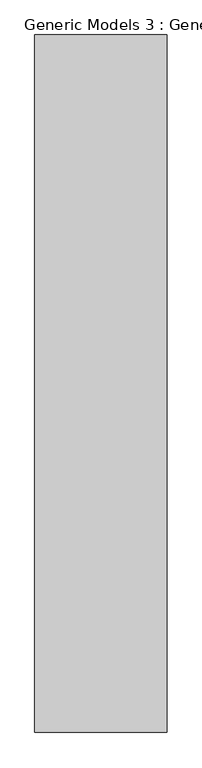
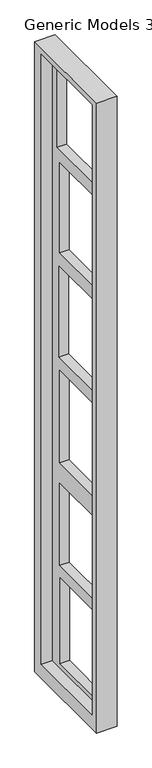
"""IFC4 building model written with IfcOpenShell, lengths in millimetres: proxy geometry, Generic Models 3 : Generic Models 1."""

from ifc_helpers import new_model, si_unit, origin, place, context, project, spatial, faceted_brep, source, transform, mapped, element, save


def generic_models_3_generic_models_1_639dc579(model_context):
    return source(origin(), model_context, "Body", "Brep", [
        faceted_brep([(-6457.5487703, -529.1037749, 18288.0), (-6457.5487703, 2442.6962251, 18288.0), (-7022.5256993, 2442.6962251, 18288.0), (-7022.5256993, -529.1037749, 18288.0), (-6457.5487703, -529.1037749, -158.4213758), (-7022.5256993, -529.1037749, -158.4213758), (-7022.5256993, 2442.6962251, -158.4213758), (-6457.5487703, 2442.6962251, -158.4213758), (-6457.5487703, 80.4962251, 15427.4465317), (-6457.5487703, 80.4962251, 17896.0910797), (-6457.5487703, 1889.1429371, 17896.0910797), (-6457.5487703, 1889.1429371, 15427.4465317), (-6457.5487703, -8.6872134, 12397.0580072), (-6457.5487703, -8.6872134, 15042.3231805), (-6457.5487703, 1781.5076359, 15042.3231805), (-6457.5487703, 1781.5076359, 12397.0580072), (-6457.5487703, -17.3853235, 9328.6434489), (-6457.5487703, -17.3853235, 11990.9234937), (-6457.5487703, 1807.8390259, 11990.9234937), (-6457.5487703, 1807.8390259, 9328.6434489), (-6457.5487703, -30.6801441, 6248.4), (-6457.5487703, -30.6801441, 8955.1024994), (-6457.5487703, 1778.1125113, 8955.1024994), (-6457.5487703, 1778.1125113, 6248.4), (-6457.5487703, -22.1772395, 3249.0844472), (-6457.5487703, -22.1772395, 5661.4894523), (-6457.5487703, 1769.7396662, 5661.4894523), (-6457.5487703, 1769.7396662, 3249.0844472), (-6457.5487703, -35.8456262, 382.1575328), (-6457.5487703, -35.8456262, 2893.6398867), (-6457.5487703, 1759.3912226, 2893.6398867), (-6457.5487703, 1759.3912226, 382.1575328), (-7022.5256993, -312.6392341, 18107.7487565), (-7022.5256993, -312.6392341, 247.1582995), (-7022.5256993, 2127.9635925, 247.1582995), (-7022.5256993, 2127.9635925, 18107.7487565), (-6717.7256993, -312.6392341, 18107.7487565), (-6717.7256993, 2127.9635925, 18107.7487565), (-6717.7256993, 2127.9635925, 247.1582995), (-6717.7256993, -312.6392341, 247.1582995), (-6717.7256993, 80.4962251, 17896.0910797), (-6717.7256993, 80.4962251, 15427.4465317), (-6717.7256993, 1889.1429371, 15427.4465317), (-6717.7256993, 1889.1429371, 17896.0910797), (-6717.7256993, -8.6872134, 15042.3231805), (-6717.7256993, -8.6872134, 12397.0580072), (-6717.7256993, 1781.5076359, 12397.0580072), (-6717.7256993, 1781.5076359, 15042.3231805), (-6717.7256993, -17.3853235, 11990.9234937), (-6717.7256993, -17.3853235, 9328.6434489), (-6717.7256993, 1807.8390259, 9328.6434489), (-6717.7256993, 1807.8390259, 11990.9234937), (-6717.7256993, -30.6801441, 8955.1024994), (-6717.7256993, -30.6801441, 6248.4), (-6717.7256993, 1778.1125113, 6248.4), (-6717.7256993, 1778.1125113, 8955.1024994), (-6717.7256993, -22.1772395, 5661.4894523), (-6717.7256993, -22.1772395, 3249.0844472), (-6717.7256993, 1769.7396662, 3249.0844472), (-6717.7256993, 1769.7396662, 5661.4894523), (-6717.7256993, -35.8456262, 2893.6398867), (-6717.7256993, -35.8456262, 382.1575328), (-6717.7256993, 1759.3912226, 382.1575328), (-6717.7256993, 1759.3912226, 2893.6398867)], [[[0, 1, 2, 3]], [[4, 5, 6, 7]], [[1, 0, 4, 7], [8, 9, 10, 11], [12, 13, 14, 15], [16, 17, 18, 19], [20, 21, 22, 23], [24, 25, 26, 27], [28, 29, 30, 31]], [[2, 1, 7, 6]], [[3, 2, 6, 5], [32, 33, 34, 35]], [[0, 3, 5, 4]], [[36, 37, 38, 39], [40, 41, 42, 43], [44, 45, 46, 47], [48, 49, 50, 51], [52, 53, 54, 55], [56, 57, 58, 59], [60, 61, 62, 63]], [[36, 39, 33, 32]], [[39, 38, 34, 33]], [[38, 37, 35, 34]], [[37, 36, 32, 35]], [[40, 9, 8, 41]], [[41, 8, 11, 42]], [[42, 11, 10, 43]], [[9, 40, 43, 10]], [[44, 13, 12, 45]], [[45, 12, 15, 46]], [[46, 15, 14, 47]], [[13, 44, 47, 14]], [[48, 17, 16, 49]], [[49, 16, 19, 50]], [[50, 19, 18, 51]], [[17, 48, 51, 18]], [[52, 21, 20, 53]], [[53, 20, 23, 54]], [[54, 23, 22, 55]], [[21, 52, 55, 22]], [[56, 25, 24, 57]], [[57, 24, 27, 58]], [[58, 27, 26, 59]], [[25, 56, 59, 26]], [[60, 29, 28, 61]], [[61, 28, 31, 62]], [[62, 31, 30, 63]], [[29, 60, 63, 30]]]),
    ])


if __name__ == "__main__":
    model = new_model("IFC4")
    model_context = context("Model", 3, world=origin())
    ifc_project = project(units=[si_unit("LENGTHUNIT", "METRE", prefix="MILLI")], contexts=[model_context])
    site = spatial("IfcSite", under=ifc_project)
    building = spatial("IfcBuilding", under=site)
    placement = place(None, origin())
    generic_models_3_generic_models_1_shape = generic_models_3_generic_models_1_639dc579(model_context)
    element("IfcBuildingElementProxy", 1, Name="Generic Models 3 : Generic Models 1", ObjectType="Generic Models 3 : Generic Models 1", at=placement, inside=building, context=model_context, shape_type="MappedRepresentation", body=[
        mapped(generic_models_3_generic_models_1_shape, transform((0.0, 0.0, 0.0), x_axis=(1.0, 0.0, 0.0), y_axis=(0.0, 1.0, 0.0), z_axis=(0.0, 0.0, 1.0))),
    ])
    save(model, "model.ifc")
